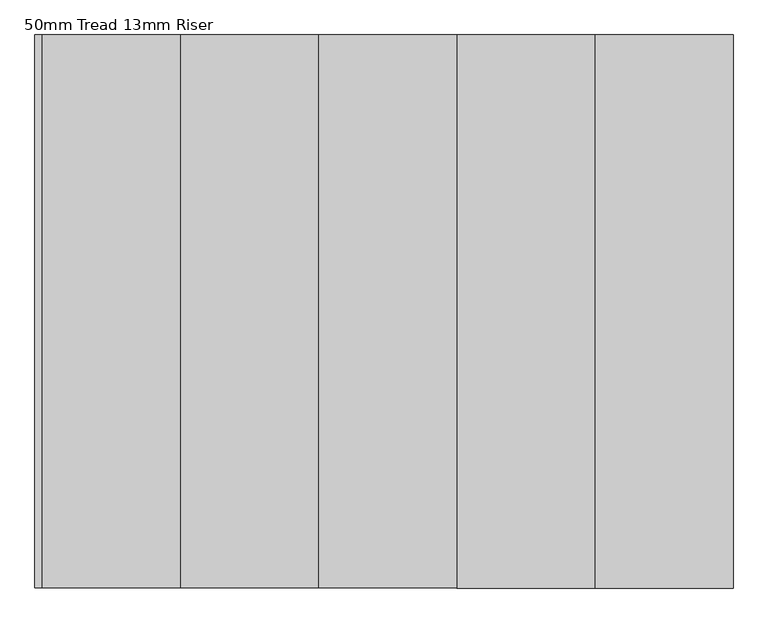
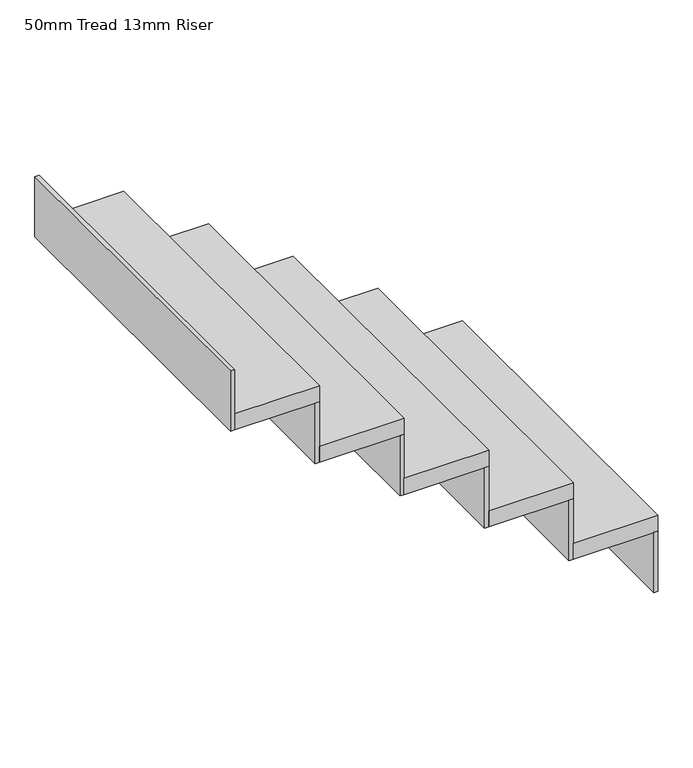
"""IFC4 building model written with IfcOpenShell, lengths in millimetres: stair flight geometry, 50mm Tread 13mm Riser."""

from ifc_helpers import new_model, si_unit, frame, origin, place, context, project, spatial, polyline, outline, extrude, source, transform, mapped, element, save


def stair_flight_50mm_tread_13mm_riser_69affff4(model_context):
    return source(origin(), model_context, "Body", "SweptSolid", [
        extrude(outline(polyline([(-10480.6794909, -3251.1360696), (-10468.1794909, -3251.1360696), (-10468.1794909, -4251.1618509), (-10480.6794909, -4251.1618509), (-10480.6794909, -3251.1360696)])), frame((0.0, 0.0, 8421.6470588), z_axis=(0.0, 0.0, 1.0), x_axis=(1.0, 0.0, 0.0)), (0.0, 0.0, 1.0), 188.2588235),
        extrude(outline(polyline([(-10718.1794909, -4251.1618509), (-10718.1794909, -3251.1360696), (-10468.1794909, -3251.1360696), (-10468.1794909, -4251.1618509), (-10718.1794909, -4251.1618509)])), frame((0.0, 0.0, 8609.9058824), z_axis=(0.0, 0.0, 1.0), x_axis=(1.0, 0.0, 0.0)), (0.0, 0.0, 1.0), 50.0),
        extrude(outline(polyline([(-10730.6794909, -3251.1360696), (-10718.1794909, -3251.1360696), (-10718.1794909, -4251.1618509), (-10730.6794909, -4251.1618509), (-10730.6794909, -3251.1360696)])), frame((0.0, 0.0, 8609.9058824), z_axis=(0.0, 0.0, 1.0), x_axis=(1.0, 0.0, 0.0)), (0.0, 0.0, 1.0), 188.2588235),
        extrude(outline(polyline([(-10968.1794909, -4251.1618509), (-10968.1794909, -3251.1360696), (-10718.1794909, -3251.1360696), (-10718.1794909, -4251.1618509), (-10968.1794909, -4251.1618509)])), frame((0.0, 0.0, 8798.1647059), z_axis=(0.0, 0.0, 1.0), x_axis=(1.0, 0.0, 0.0)), (0.0, 0.0, 1.0), 50.0),
        extrude(outline(polyline([(-10980.6794909, -3251.1360696), (-10968.1794909, -3251.1360696), (-10968.1794909, -4251.1618509), (-10980.6794909, -4251.1618509), (-10980.6794909, -3251.1360696)])), frame((0.0, 0.0, 8798.1647059), z_axis=(0.0, 0.0, 1.0), x_axis=(1.0, 0.0, 0.0)), (0.0, 0.0, 1.0), 188.2588235),
        extrude(outline(polyline([(-11218.1794909, -4251.1618509), (-11218.1794909, -3251.1360696), (-10968.1794909, -3251.1360696), (-10968.1794909, -4251.1618509), (-11218.1794909, -4251.1618509)])), frame((0.0, 0.0, 8986.4235294), z_axis=(0.0, 0.0, 1.0), x_axis=(1.0, 0.0, 0.0)), (0.0, 0.0, 1.0), 50.0),
        extrude(outline(polyline([(-11230.6794909, -3251.1360696), (-11218.1794909, -3251.1360696), (-11218.1794909, -4251.1618509), (-11230.6794909, -4251.1618509), (-11230.6794909, -3251.1360696)])), frame((0.0, 0.0, 8986.4235294), z_axis=(0.0, 0.0, 1.0), x_axis=(1.0, 0.0, 0.0)), (0.0, 0.0, 1.0), 188.2588235),
        extrude(outline(polyline([(-11468.1794909, -4251.1618509), (-11468.1794909, -3251.1360696), (-11218.1794909, -3251.1360696), (-11218.1794909, -4251.1618509), (-11468.1794909, -4251.1618509)])), frame((0.0, 0.0, 9174.6823529), z_axis=(0.0, 0.0, 1.0), x_axis=(1.0, 0.0, 0.0)), (0.0, 0.0, 1.0), 50.0),
        extrude(outline(polyline([(-11480.6794909, -3251.1360696), (-11468.1794909, -3251.1360696), (-11468.1794909, -4251.1618509), (-11480.6794909, -4251.1618509), (-11480.6794909, -3251.1360696)])), frame((0.0, 0.0, 9174.6823529), z_axis=(0.0, 0.0, 1.0), x_axis=(1.0, 0.0, 0.0)), (0.0, 0.0, 1.0), 188.2588235),
        extrude(outline(polyline([(-11730.6794909, -3251.1360696), (-11718.1794909, -3251.1360696), (-11718.1794909, -4251.1618509), (-11730.6794909, -4251.1618509), (-11730.6794909, -3251.1360696)])), frame((0.0, 0.0, 9362.9411765), z_axis=(0.0, 0.0, 1.0), x_axis=(1.0, 0.0, 0.0)), (0.0, 0.0, 1.0), 188.2588235),
        extrude(outline(polyline([(-11718.1794909, -4251.1618509), (-11718.1794909, -3251.1360696), (-11468.1794909, -3251.1360696), (-11468.1794909, -4251.1618509), (-11718.1794909, -4251.1618509)])), frame((0.0, 0.0, 9362.9411765), z_axis=(0.0, 0.0, 1.0), x_axis=(1.0, 0.0, 0.0)), (0.0, 0.0, 1.0), 50.0),
    ])


if __name__ == "__main__":
    model = new_model("IFC4")
    model_context = context("Model", 3, world=origin())
    ifc_project = project(units=[si_unit("LENGTHUNIT", "METRE", prefix="MILLI")], contexts=[model_context])
    site = spatial("IfcSite", under=ifc_project)
    building = spatial("IfcBuilding", under=site)
    placement = place(None, origin())
    stair_flight_50mm_tread_13mm_riser_shape = stair_flight_50mm_tread_13mm_riser_69affff4(model_context)
    element("IfcStairFlight", 1, ObjectType="50mm Tread 13mm Riser", at=placement, inside=building, context=model_context, shape_type="MappedRepresentation", body=[
        mapped(stair_flight_50mm_tread_13mm_riser_shape, transform((0.0, 0.0, 0.0), x_axis=(1.0, 0.0, 0.0), y_axis=(0.0, 1.0, 0.0), z_axis=(0.0, 0.0, 1.0))),
    ])
    save(model, "model.ifc")
